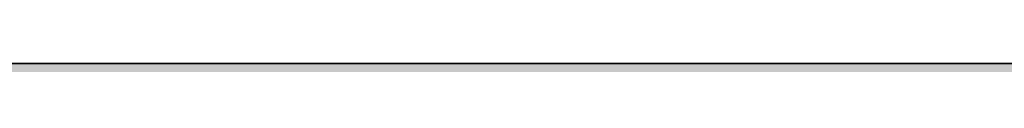
# Model space of a CAD drawing. Units: inches. Extents: x 2091 to 2899, y 967 to 2217.
# Tile 58 of 256: x 2212.16216 to 2212.20615, y 1099.919 to 1099.91906. Entities that reach past the tile are written whole.
import ezdxf

# ---------------------------------------------------------------- set-up
doc = ezdxf.new("R2010")
doc.units = ezdxf.units.IN
doc.layers.add('A-WALL-PATT', color=141, linetype='Continuous', lineweight=13, true_color=0xadddf7)
doc.layers.add('L-SITE-WALL', color=7, linetype='Continuous', lineweight=35)

msp = doc.modelspace()

# ---------------------------------------------------------------- hatches: boundary and pattern name
at = {"layer": 'A-WALL-PATT'}
h = msp.add_hatch(color=256, dxfattribs=at)
h.dxf.hatch_style = 1
h.paths.add_polyline_path([(2212.143603, 1941.419059), (2387.643603, 1941.419059), (2387.643603, 1824.419059), (2392.143603, 1824.419059), (2392.143603, 1941.419059), (2609.643603, 1941.419059), (2609.643603, 1825.919059), (2614.143603, 1825.919059), (2614.143603, 1941.419059), (2794.143603, 1941.419059), (2794.143603, 1928.762166), (2803.143603, 1928.762166), (2803.143603, 2050.919059), (2203.143603, 2050.919059), (2203.143603, 1900.757859), (2212.143603, 1900.757859)])
h.paths.add_polyline_path([(2212.143603, 1945.919059), (2212.143603, 2041.919059), (2794.143603, 2041.919059), (2794.143603, 1945.919059), (2402.248245, 1945.919059), (2401.102434, 1945.775832), (2398.702434, 1945.775832)], flags=16)
h.paths.add_polyline_path([(2230.229861, 1948.062793), (2227.349861, 1949.502793), (2225.909861, 1951.902793), (2223.989861, 1952.862793), (2223.029861, 1955.262793), (2222.069861, 1959.582793), (2222.069861, 1963.422793), (2223.029861, 1965.662793), (2223.989861, 1965.342793), (2225.58591, 1963.860747), (2226.911533, 1964.957259), (2226.948861, 1965.938793), (2227.778319, 1966.952143), (2228.199916, 1968.878704), (2230.709861, 1964.862793), (2233.589861, 1966.302793), (2233.607309, 1966.331873), (2233.772659, 1964.938205), (2234.633802, 1963.676473), (2235.029861, 1963.902793), (2236.282035, 1965.572358), (2235.989861, 1962.942793), (2237.954512, 1957.540002), (2238.389861, 1957.902793), (2239.215861, 1960.305793), (2238.654565, 1966.38496), (2238.692792, 1966.438069), (2238.840578, 1967.499707), (2238.780291, 1967.687486), (2238.880538, 1967.786763), (2238.666861, 1966.251793), (2239.215861, 1960.305793), (2238.389861, 1957.902793), (2236.949861, 1956.702793), (2234.549861, 1949.982793)], flags=0)
h.paths.add_polyline_path([(2278.011974, 1948.062793), (2276.496427, 1947.873349), (2275.849833, 1947.688608), (2274.651974, 1947.102793)], flags=0)
h.paths.add_polyline_path([(2269.851974, 1955.742793), (2268.276176, 1956.629329), (2270.867302, 1956.348398), (2269.371974, 1958.142793), (2268.714964, 1959.192325), (2270.569833, 1958.728608), (2268.580725, 1961.906087), (2270.811974, 1960.891883), (2270.811974, 1963.422793), (2271.393315, 1964.779256), (2270.291762, 1966.156196), (2271.771974, 1965.662793), (2272.141387, 1966.524757), (2273.929833, 1965.928608), (2275.630385, 1968.054299), (2276.331938, 1966.72186), (2276.520431, 1966.952143), (2276.942029, 1968.878704), (2277.734293, 1967.611082), (2278.139888, 1969.46452), (2279.659124, 1967.033742), (2280.411974, 1966.782793), (2280.949302, 1967.588785), (2281.609833, 1967.368608), (2282.133266, 1968.153758), (2282.349235, 1966.333445), (2282.349849, 1966.332585), (2283.40755, 1968.09542), (2283.712631, 1965.52402), (2284.320221, 1964.633789), (2284.511809, 1964.889239), (2284.234974, 1965.704793), (2284.500472, 1967.318958), (2284.907944, 1965.41742), (2285.396313, 1966.068579), (2285.432833, 1966.290608), (2285.473338, 1966.171279), (2286.353919, 1967.345387), (2286.222007, 1966.158173), (2287.663492, 1968.080154), (2287.713974, 1968.442793), (2288.481599, 1969.016679), (2288.573993, 1968.728897), (2288.917461, 1969.06904), (2288.606833, 1966.837608), (2288.928726, 1963.35131), (2288.934974, 1963.356793), (2288.929731, 1963.340422), (2289.015281, 1962.413869), (2290.111223, 1963.875126), (2290.132833, 1963.942608), (2290.217672, 1964.017058), (2290.111223, 1963.875126), (2289.155833, 1960.891608), (2288.594036, 1959.257227), (2288.571974, 1959.102793), (2289.531974, 1960.542793), (2290.011974, 1962.462793), (2290.19184, 1962.642659), (2289.769833, 1959.688608), (2286.889833, 1957.288608), (2284.489833, 1950.568608), (2283.314658, 1950.046308), (2283.291974, 1949.982793), (2280.290059, 1948.648608), (2281.129833, 1948.648608), (2282.569833, 1948.168608), (2283.204726, 1948.062793), (2278.971974, 1948.062793), (2276.091974, 1949.502793), (2274.651974, 1951.902793), (2272.731974, 1952.862793)], flags=0)
h.paths.add_polyline_path([(2271.158868, 1958.021765), (2272.969833, 1955.848608), (2272.009833, 1960.168608), (2272.009833, 1964.008608), (2272.624426, 1965.442658), (2274.328023, 1963.860747), (2275.653646, 1964.957259), (2275.637743, 1964.53909), (2277.412231, 1966.006888), (2277.032974, 1965.156793), (2276.829924, 1964.975597), (2276.766012, 1963.295014), (2277.449635, 1962.66022), (2279.451974, 1964.862793), (2282.331974, 1966.302793), (2283.529833, 1966.888608), (2283.294512, 1966.770948), (2283.912993, 1963.8847), (2284.899249, 1964.448275), (2284.731974, 1962.942793), (2286.696625, 1957.540002), (2287.131974, 1957.902793), (2287.541913, 1959.095388), (2287.779395, 1958.442311), (2285.682738, 1956.695097), (2285.876503, 1959.795336), (2284.731974, 1962.942793), (2284.899249, 1964.448275), (2283.912993, 1963.8847), (2284.223833, 1962.434116), (2283.424365, 1963.605484), (2281.609833, 1962.568608), (2281.129833, 1960.168608), (2282.089833, 1956.328608), (2283.049833, 1952.968608), (2282.569833, 1950.568608), (2280.169833, 1948.648608), (2279.883316, 1948.791867), (2278.971974, 1948.062793), (2278.971974, 1949.022793), (2278.672313, 1949.397368), (2277.289833, 1950.088608), (2275.849833, 1952.488608), (2273.929833, 1953.448608), (2272.489833, 1954.888608), (2271.921647, 1954.888608), (2271.771974, 1955.262793)], flags=0)
h.paths.add_polyline_path([(2311.994146, 1955.742793), (2312.062717, 1955.674221), (2312.0551, 1955.7085)], flags=0)
h.paths.add_polyline_path([(2331.956146, 1963.951793), (2333.396146, 1965.391793), (2331.077146, 1963.356793), (2330.998603, 1963.111517)], flags=0)
h.paths.add_polyline_path([(2310.554146, 1954.302793), (2307.039807, 1956.279943), (2310.762903, 1955.876284), (2312.474146, 1953.822793), (2313.434146, 1951.422793), (2315.354146, 1950.462793), (2316.794146, 1948.062793), (2317.466146, 1947.726793), (2319.368691, 1947.964611), (2317.754146, 1949.982793), (2317.569531, 1950.610485), (2316.794146, 1951.902793), (2314.874146, 1952.862793), (2313.914146, 1955.262793), (2311.514146, 1958.142793), (2309.375489, 1961.559168), (2311.514146, 1960.337078), (2311.514146, 1961.982793), (2310.604672, 1963.119635), (2311.726605, 1962.47853), (2312.418332, 1964.09256), (2312.255964, 1964.29552), (2313.194146, 1963.982793), (2313.914146, 1965.662793), (2314.646778, 1965.418582), (2315.354146, 1966.302793), (2316.794146, 1967.742793), (2316.157435, 1966.946904), (2317.034111, 1965.28186), (2317.222604, 1965.512143), (2317.777048, 1968.045771), (2318.474111, 1966.72186), (2318.662604, 1966.952143), (2319.084201, 1968.878704), (2321.207049, 1965.482147), (2322.161419, 1966.913702), (2322.554146, 1966.782793), (2322.785988, 1967.130555), (2322.881646, 1966.324293), (2323.312041, 1965.72174), (2323.651289, 1965.891364), (2324.3965, 1967.133382), (2324.656945, 1964.938205), (2324.971986, 1964.476611), (2325.38728, 1967.001499), (2325.940813, 1964.418348), (2327.228929, 1966.135836), (2327.16632, 1965.572358), (2328.059139, 1966.762783), (2328.224576, 1966.247486), (2329.667971, 1967.67691), (2329.664576, 1967.687486), (2329.764823, 1967.786763), (2329.551146, 1966.251793), (2330.100146, 1960.305793), (2329.332814, 1958.07347), (2329.313065, 1957.935225), (2329.634146, 1958.202793), (2330.234146, 1959.102793), (2330.714146, 1961.022793), (2331.034146, 1961.342793), (2330.714146, 1959.102793), (2329.634146, 1958.202793), (2329.274146, 1957.662793), (2327.712112, 1956.361098), (2325.434146, 1949.982793), (2324.333769, 1949.493736), (2323.994146, 1948.542793), (2319.674146, 1946.622793), (2316.794146, 1948.062793), (2315.354146, 1950.462793), (2313.434146, 1951.422793)], flags=0)
h.paths.add_polyline_path([(2321.335684, 1947.952023), (2321.114146, 1948.062793), (2321.114146, 1949.022793), (2319.194146, 1951.422793), (2316.794146, 1959.582793), (2316.663237, 1959.582793), (2315.354146, 1958.142793), (2314.394146, 1958.142793), (2313.148303, 1958.709085), (2312.954146, 1959.582793), (2312.954146, 1960.891883), (2315.834146, 1959.582793), (2316.663237, 1959.582793), (2317.314709, 1960.299412), (2315.030195, 1962.420747), (2316.355818, 1963.517259), (2316.372337, 1963.951615), (2316.470195, 1963.860747), (2317.795818, 1964.957259), (2317.755219, 1963.889687), (2319.175146, 1965.156793), (2319.498407, 1965.881372), (2321.114146, 1965.342793), (2323.235885, 1962.372358), (2325.686349, 1963.772623), (2325.542789, 1962.480576), (2325.198783, 1963.494014), (2324.47851, 1963.082429), (2324.926005, 1960.994116), (2324.078087, 1962.236473), (2322.414791, 1961.286018), (2322.074146, 1959.582793), (2323.034146, 1955.742793), (2323.994146, 1952.382793), (2323.514146, 1949.982793), (2322.142717, 1948.88565), (2322.074146, 1948.542793)], flags=0)
h.paths.add_polyline_path([(2320.207479, 1963.337459), (2320.154146, 1963.422793), (2320.394146, 1963.542793)], flags=0)
h.paths.add_polyline_path([(2353.850527, 1965.8105), (2354.030527, 1965.7505), (2354.330527, 1966.4505), (2354.330527, 1966.9305)], flags=0)
h.paths.add_polyline_path([(2359.020582, 1969.026412), (2359.098382, 1968.901932), (2359.233527, 1969.5195), (2359.233527, 1969.9995)], flags=0)
h.paths.add_polyline_path([(2358.256694, 1966.681672), (2357.983601, 1966.348035), (2358.211267, 1966.146175), (2358.410492, 1966.389568)], flags=0)
h.paths.add_polyline_path([(2357.768473, 1966.058778), (2357.7322, 1965.104967), (2357.751047, 1965.120556), (2357.769527, 1965.6065), (2357.769527, 1966.057843)], flags=0)
h.paths.add_polyline_path([(2359.111527, 1965.3045), (2359.111527, 1964.8245), (2359.844527, 1966.4675), (2359.844527, 1966.9475)], flags=0)
h.paths.add_polyline_path([(2360.223684, 1966.621449), (2360.698527, 1969.3625), (2360.698527, 1969.8425), (2360.210527, 1967.0255), (2360.210527, 1966.6425)], flags=0)
h.paths.add_polyline_path([(2363.450527, 1967.8905), (2363.450527, 1968.3705), (2362.490527, 1966.9305), (2362.656045, 1966.698776)], flags=0)
h.paths.add_polyline_path([(2364.475523, 1966.078826), (2365.850527, 1968.3705), (2365.850527, 1968.8505), (2364.427975, 1966.479581)], flags=0)
h.paths.add_polyline_path([(2366.313527, 1965.8525), (2366.366709, 1965.695829), (2366.802527, 1968.3455), (2366.802527, 1968.8255)], flags=0)
h.paths.add_polyline_path([(2367.16531, 1965.803544), (2367.290527, 1966.9305), (2367.290527, 1967.4105), (2367.102701, 1965.720066)], flags=0)
h.paths.add_polyline_path([(2370.036527, 1959.9735), (2371.013527, 1963.0245), (2371.013527, 1963.5045), (2370.036527, 1960.4535)], flags=0)
h.paths.add_polyline_path([(2371.610527, 1960.2105), (2372.570527, 1961.6505), (2372.570527, 1962.1305), (2371.802527, 1960.9785)], flags=0)
h.paths.add_polyline_path([(2350.873666, 1956.005086), (2351.930527, 1955.8905), (2354.490527, 1953.3305), (2353.850527, 1954.9305), (2351.450527, 1957.8105), (2347.935527, 1963.4255), (2347.935527, 1963.9055), (2351.450527, 1958.2905), (2353.705073, 1955.585046), (2352.890527, 1959.2505), (2352.890527, 1959.7305), (2352.890527, 1961.924786), (2356.730527, 1959.7305), (2358.454471, 1961.626838), (2354.810527, 1965.0105), (2355.030855, 1965.28591), (2358.691091, 1961.88712), (2361.530527, 1965.0105), (2364.376495, 1966.433484), (2364.524394, 1965.186911), (2365.454468, 1963.824181), (2365.881073, 1964.067955), (2365.370527, 1966.4505), (2365.370527, 1966.9305), (2366.810527, 1960.2105), (2366.810527, 1959.7305), (2366.388709, 1952.981409), (2367.770527, 1956.8505), (2368.641225, 1957.576082), (2366.810527, 1962.6105), (2366.810527, 1963.0905), (2368.775179, 1957.68771), (2369.210527, 1958.0505), (2370.001592, 1960.351867), (2369.475232, 1966.052668), (2369.513458, 1966.105777), (2369.514173, 1966.110912), (2369.475232, 1966.532668), (2369.513458, 1966.585777), (2369.614635, 1967.312591), (2369.182527, 1968.6585), (2369.182527, 1969.1385), (2369.600957, 1967.835194), (2369.701204, 1967.934471), (2369.717947, 1968.054743), (2370.145176, 1968.374145), (2369.778707, 1968.011224), (2369.701204, 1967.454471), (2370.468161, 1968.214004), (2369.674936, 1967.265771), (2369.514173, 1966.110912), (2370.036527, 1960.4535), (2370.036527, 1959.9735), (2369.441756, 1958.243191), (2370.650527, 1959.2505), (2371.045821, 1962.017559), (2371.130527, 1962.1305), (2370.650527, 1958.7705), (2367.770527, 1956.3705), (2365.370527, 1949.6505), (2362.079099, 1948.187643), (2363.450527, 1947.7305), (2361.050527, 1947.7305), (2360.090527, 1947.7305), (2357.103861, 1947.357167), (2360.090527, 1948.2105), (2358.170527, 1949.1705), (2356.730527, 1951.5705), (2354.810527, 1952.5305), (2351.930527, 1955.4105)], flags=0)
h.paths.add_polyline_path([(2361.050527, 1948.6905), (2359.130527, 1951.0905), (2356.730527, 1959.2505), (2355.770527, 1959.2505), (2352.890527, 1960.559591), (2352.890527, 1961.444786), (2355.890527, 1959.7305), (2356.730527, 1959.7305), (2356.837194, 1959.367834), (2361.530527, 1964.5305), (2363.248422, 1965.389448), (2364.92531, 1963.041805), (2362.490527, 1961.6505), (2362.063861, 1959.517167), (2362.970527, 1955.8905), (2363.930527, 1952.5305), (2363.930527, 1952.0505), (2363.450527, 1949.6505), (2361.050527, 1947.7305)], flags=0)
h.paths.add_polyline_path([(2359.130527, 1951.5705), (2359.290527, 1951.3705), (2361.050527, 1954.4505), (2361.050527, 1954.9305)], flags=0)
h.paths.add_polyline_path([(2357.219527, 1966.5455), (2356.792527, 1968.8145), (2356.792527, 1969.2945), (2357.219527, 1967.0255)], flags=0)
h.paths.add_polyline_path([(2361.050527, 1954.4505), (2361.530527, 1958.7705), (2361.530527, 1959.2505), (2361.050527, 1954.9305)], flags=0)
h.paths.add_polyline_path([(2402.548287, 1948.486076), (2402.302434, 1948.415832), (2402.590434, 1948.415832)], flags=0)
h.paths.add_polyline_path([(2394.142434, 1956.095832), (2395.685052, 1954.553214), (2396.720495, 1953.970679), (2396.062434, 1955.615832), (2395.241381, 1956.601096), (2395.878904, 1956.441715), (2395.102434, 1959.935832), (2395.102434, 1963.775832), (2396.062434, 1966.015832), (2397.022434, 1965.695832), (2398.618483, 1964.213787), (2399.944106, 1965.310299), (2399.981434, 1966.291832), (2400.810891, 1967.305183), (2401.232489, 1969.231744), (2403.537949, 1965.543008), (2403.941984, 1967.389316), (2404.702434, 1967.135832), (2405.460328, 1966.07478), (2406.622434, 1966.655832), (2406.639882, 1966.684913), (2406.805232, 1965.291245), (2406.925694, 1965.114746), (2407.342434, 1964.975832), (2407.874326, 1965.77367), (2408.1691, 1964.398055), (2409.314608, 1965.925398), (2409.217458, 1965.051054), (2409.445232, 1963.131245), (2410.306374, 1961.869513), (2410.702434, 1962.095832), (2411.442269, 1963.082279), (2411.165434, 1963.897832), (2411.616426, 1966.639757), (2411.725365, 1966.791109), (2411.873151, 1967.852747), (2411.812864, 1968.040526), (2411.913111, 1968.139803), (2411.699434, 1966.604832), (2412.248434, 1960.658832), (2413.225434, 1963.709832), (2414.3779, 1964.72116), (2414.513151, 1965.692747), (2414.452864, 1965.880526), (2414.553111, 1965.979803), (2414.3779, 1964.72116), (2414.519817, 1964.845697), (2414.365365, 1964.631109), (2414.339434, 1964.444832), (2414.888434, 1958.498832), (2414.062434, 1956.095832), (2412.622434, 1954.895832), (2410.17137, 1948.032854), (2410.016719, 1948.084404), (2405.902434, 1946.255832), (2405.902434, 1947.215832), (2405.204252, 1948.08856), (2404.222434, 1948.415832), (2403.262434, 1948.415832), (2400.382434, 1949.855832), (2399.662434, 1951.055832), (2397.982434, 1952.735832), (2397.022434, 1953.215832), (2395.685052, 1954.553214), (2392.656776, 1956.256908)], flags=0)
h.paths.add_polyline_path([(2409.08565, 1964.407441), (2409.130363, 1964.275715), (2409.262434, 1964.495832)], flags=0)
h.paths.add_polyline_path([(2397.742434, 1961.615832), (2398.702434, 1963.855832), (2399.662434, 1963.535832), (2401.426563, 1965.740994), (2401.791415, 1966.5588), (2402.071434, 1965.070832), (2402.835507, 1964.393367), (2403.262398, 1964.9149), (2403.338119, 1964.771086), (2402.615516, 1963.976223), (2402.498612, 1960.902238), (2403.542997, 1959.932452), (2404.413203, 1960.889679), (2404.702434, 1962.335832), (2407.916347, 1964.172354), (2409.520211, 1961.926944), (2410.987085, 1957.893042), (2411.422434, 1958.255832), (2412.047964, 1960.075625), (2412.410341, 1959.079088), (2411.675621, 1958.466821), (2411.662434, 1958.255832), (2411.62607, 1958.425529), (2409.982434, 1957.055832), (2407.582434, 1950.335832), (2403.262434, 1948.415832), (2403.262434, 1949.375832), (2401.342434, 1951.775832), (2399.416508, 1958.323981), (2397.742434, 1959.084923), (2397.742434, 1959.970118), (2397.102434, 1960.335832), (2397.742434, 1960.044923)], flags=0)
h.paths.add_polyline_path([(2405.902434, 1952.975832), (2405.950434, 1953.407832), (2406.016719, 1953.175832)], flags=0)
h.paths.add_polyline_path([(2449.817778, 1967.114014), (2449.752323, 1967.135832), (2449.793703, 1967.077901)], flags=0)
h.paths.add_polyline_path([(2451.697696, 1966.61812), (2451.740895, 1966.690118), (2451.692051, 1966.665696)], flags=0)
h.paths.add_polyline_path([(2454.343628, 1965.737572), (2455.752323, 1967.615832), (2455.992323, 1968.095832), (2454.364497, 1965.925398)], flags=0)
h.paths.add_polyline_path([(2457.547323, 1968.863832), (2457.787323, 1969.343832), (2457.054323, 1968.795832), (2457.007622, 1968.460345)], flags=0)
h.paths.add_polyline_path([(2456.921784, 1967.856662), (2456.802238, 1968.229016), (2456.723, 1967.659803)], flags=0)
h.paths.add_polyline_path([(2457.302323, 1967.376832), (2457.542323, 1967.856832), (2456.810323, 1966.839832), (2456.740516, 1966.700218), (2456.749021, 1966.608105)], flags=0)
h.paths.add_polyline_path([(2458.275323, 1963.709832), (2458.155343, 1963.335153), (2460.354323, 1965.264832), (2460.594323, 1965.744832)], flags=0)
h.paths.add_polyline_path([(2458.392323, 1962.815832), (2458.364088, 1962.618185), (2459.592323, 1964.255832), (2459.832323, 1964.735832)], flags=0)
h.paths.add_polyline_path([(2459.352323, 1962.815832), (2459.272323, 1962.495832), (2460.072323, 1963.295832), (2460.312323, 1963.775832)], flags=0)
h.paths.add_polyline_path([(2458.680323, 1960.607832), (2458.632323, 1960.415832), (2459.592323, 1961.855832), (2459.832323, 1962.335832)], flags=0)
h.paths.add_polyline_path([(2437.83817, 1956.24265), (2439.192323, 1956.095832), (2441.352323, 1953.935832), (2440.872323, 1955.135832), (2438.472323, 1958.015832), (2438.071563, 1958.656023), (2438.712323, 1958.495832), (2440.639596, 1956.183105), (2439.912323, 1959.455832), (2439.912323, 1963.295832), (2441.352323, 1966.655832), (2441.592323, 1967.135832), (2441.112323, 1966.015832), (2442.072323, 1965.695832), (2443.988993, 1968.09167), (2444.241323, 1966.750832), (2444.916801, 1966.15192), (2445.676574, 1967.080136), (2446.255323, 1969.724832), (2446.495323, 1970.204832), (2446.282379, 1969.231744), (2447.362672, 1967.503275), (2447.720323, 1969.567832), (2447.960323, 1970.047832), (2447.48548, 1967.306781), (2448.792323, 1965.215832), (2448.472323, 1964.863832), (2448.552323, 1964.735832), (2451.452051, 1966.185696), (2451.615122, 1964.811245), (2452.307917, 1963.796172), (2453.234505, 1964.325651), (2454.072323, 1960.415832), (2453.628687, 1953.317651), (2454.792323, 1956.575832), (2455.032323, 1957.055832), (2455.718835, 1957.627926), (2453.832323, 1962.815832), (2453.940966, 1963.793615), (2453.335323, 1965.577832), (2453.824323, 1968.550832), (2454.064323, 1969.030832), (2453.575323, 1966.057832), (2454.040333, 1964.687919), (2453.832323, 1962.815832), (2455.718835, 1957.627926), (2456.367207, 1958.168235), (2457.058323, 1960.178832), (2457.298323, 1960.658832), (2456.472323, 1958.255832), (2457.717729, 1959.29367), (2457.672323, 1958.975832), (2454.889951, 1956.657188), (2453.614142, 1953.084923), (2453.592323, 1952.735832), (2453.352323, 1952.255832), (2453.359596, 1952.372196), (2452.632323, 1950.335832), (2452.392323, 1949.855832), (2449.203752, 1948.43869), (2450.712323, 1947.935832), (2448.072323, 1947.935832), (2447.112323, 1947.935832), (2444.552323, 1947.615832), (2447.199596, 1948.372196), (2445.192323, 1949.375832), (2443.752323, 1951.775832), (2441.832323, 1952.735832), (2438.952323, 1955.615832)], flags=0)
h.paths.add_polyline_path([(2443.992323, 1959.935832), (2444.040323, 1959.772632), (2444.121554, 1959.861986)], flags=0)
h.paths.add_polyline_path([(2442.912323, 1959.935832), (2443.032323, 1959.935832), (2442.445657, 1960.202499)], flags=0)
h.paths.add_polyline_path([(2444.982943, 1965.019677), (2445.279323, 1965.264832), (2445.519323, 1965.744832), (2444.993996, 1965.310299)], flags=0)
h.paths.add_polyline_path([(2446.133323, 1965.029832), (2446.330366, 1965.471499), (2444.970323, 1964.257832), (2444.730323, 1963.777832)], flags=0)
h.paths.add_polyline_path([(2442.792323, 1959.455832), (2443.752323, 1959.455832), (2446.152323, 1951.295832), (2446.412323, 1951.750832), (2446.392323, 1951.775832), (2448.080599, 1954.730315), (2448.552323, 1958.975832), (2441.832323, 1965.215832), (2442.154946, 1965.619111), (2448.792323, 1959.455832), (2448.312323, 1955.135832), (2448.072323, 1954.655832), (2446.412323, 1951.750832), (2448.312323, 1949.375832), (2448.312323, 1948.415832), (2450.540895, 1950.19869), (2450.952323, 1952.255832), (2449.992323, 1955.615832), (2449.032323, 1959.455832), (2449.512323, 1961.855832), (2449.752323, 1962.335832), (2449.674904, 1961.948736), (2452.994505, 1963.845651), (2453.064414, 1963.519409), (2452.884611, 1963.782854), (2449.674904, 1961.948736), (2449.272323, 1959.935832), (2450.232323, 1956.095832), (2451.192323, 1952.735832), (2450.712323, 1950.335832), (2450.472323, 1949.855832), (2448.072323, 1947.935832), (2448.072323, 1948.535832), (2445.432323, 1949.855832), (2443.992323, 1952.255832), (2442.072323, 1953.215832), (2441.112323, 1955.615832), (2440.152323, 1959.935832), (2440.152323, 1960.655832)], flags=0)
h.paths.add_polyline_path([(2456.692323, 1966.985832), (2457.608323, 1968.080832), (2457.848323, 1968.560832), (2456.932323, 1967.465832)], flags=0)
h.paths.add_polyline_path([(2489.89657, 1966.580241), (2489.942948, 1966.189347), (2490.747488, 1967.530248), (2491.319122, 1968.951161)], flags=0)
h.paths.add_polyline_path([(2473.562471, 1956.407131), (2477.139981, 1956.019257), (2476.955333, 1956.240834), (2475.108049, 1957.280108), (2476.347488, 1956.970248), (2475.186901, 1958.824216), (2476.919122, 1958.391161), (2475.411642, 1960.799269), (2477.787488, 1959.719339), (2477.787488, 1962.250248), (2477.637399, 1962.43786), (2477.82255, 1962.332059), (2478.359122, 1963.58406), (2478.359122, 1963.671161), (2477.324348, 1964.964628), (2478.714826, 1964.501135), (2479.319122, 1965.911161), (2480.279122, 1965.591161), (2481.783965, 1967.472214), (2482.116488, 1965.705248), (2482.880562, 1965.027782), (2483.209305, 1965.429408), (2483.220169, 1965.71509), (2483.07594, 1965.989022), (2483.711762, 1966.765808), (2484.130488, 1968.679248), (2484.702122, 1970.100161), (2484.489177, 1969.127072), (2486.502904, 1965.905109), (2487.387488, 1965.610248), (2488.153419, 1966.759144), (2488.717017, 1965.970108), (2489.200086, 1966.211642), (2489.330671, 1965.110992), (2490.393905, 1963.622465), (2490.660765, 1963.774956), (2490.493905, 1964.553636), (2490.923063, 1963.924841), (2491.319122, 1964.151161), (2491.333389, 1964.170183), (2491.210488, 1964.532248), (2491.281756, 1964.965537), (2491.425789, 1964.293383), (2494.076476, 1967.827632), (2494.497918, 1966.514942), (2494.598165, 1966.614218), (2494.689488, 1967.270248), (2495.106748, 1967.582196), (2495.129839, 1967.748075), (2495.069552, 1967.935854), (2495.169799, 1968.035131), (2495.031777, 1967.043632), (2495.753818, 1967.758684), (2494.982053, 1966.686437), (2494.956122, 1966.500161), (2495.479021, 1960.836851), (2495.910488, 1962.184248), (2496.482122, 1963.605161), (2496.072694, 1962.326589), (2496.768904, 1962.937536), (2496.599122, 1962.711161), (2496.119122, 1959.351161), (2496.732873, 1960.271787), (2496.987488, 1961.290248), (2497.559122, 1962.711161), (2497.079122, 1960.791161), (2496.507488, 1959.370248), (2495.547488, 1957.930248), (2492.758842, 1955.606376), (2490.839122, 1950.231161), (2490.267488, 1948.810248), (2485.947488, 1946.890248), (2483.067488, 1948.330248), (2481.627488, 1950.730248), (2479.707488, 1951.690248), (2476.827488, 1954.570248)], flags=0)
h.paths.add_polyline_path([(2485.576973, 1948.313392), (2485.559122, 1948.311161), (2485.578758, 1948.311161)], flags=0)
h.paths.add_polyline_path([(2478.645063, 1954.551161), (2478.109042, 1956.963257), (2479.319122, 1955.511161), (2480.279122, 1953.111161), (2482.199122, 1952.151161), (2483.639122, 1949.751161), (2486.519122, 1948.311161), (2486.519122, 1949.271161), (2484.739307, 1951.49593), (2484.027488, 1950.250248), (2481.627488, 1958.410248), (2482.375148, 1959.232673), (2482.199122, 1959.831161), (2483.197572, 1960.929456), (2479.707488, 1964.170248), (2480.603358, 1965.290085), (2481.875171, 1964.109115), (2482.666387, 1964.763582), (2482.615359, 1963.421798), (2482.989199, 1963.074661), (2484.008488, 1963.984248), (2484.683606, 1965.497507), (2484.580122, 1965.405161), (2485.357268, 1967.147113), (2485.120645, 1965.781197), (2486.427488, 1963.690248), (2488.145383, 1964.549195), (2489.822271, 1962.201552), (2490.747488, 1962.730248), (2491.999662, 1964.399813), (2492.076046, 1965.087265), (2492.212892, 1964.684119), (2492.485374, 1965.047429), (2492.279122, 1963.191161), (2494.243773, 1957.78837), (2494.562503, 1958.053978), (2494.933488, 1959.133248), (2495.505122, 1960.554161), (2494.679122, 1958.151161), (2494.107488, 1956.730248), (2494.562503, 1958.053978), (2493.408544, 1957.092345), (2491.707488, 1961.770248), (2491.999662, 1964.399813), (2490.747488, 1962.730248), (2487.71203, 1960.9957), (2487.479122, 1959.831161), (2488.439122, 1955.991161), (2489.399122, 1952.631161), (2488.919122, 1950.231161), (2488.576918, 1949.957397), (2488.347488, 1948.810248), (2487.651715, 1948.253629), (2487.479122, 1948.311161), (2486.519122, 1948.311161), (2483.639122, 1949.751161), (2482.199122, 1952.151161), (2480.279122, 1953.111161), (2478.839122, 1954.551161)], flags=0)
h.paths.add_polyline_path([(2526.648252, 1966.987524), (2526.517343, 1967.031161), (2526.600102, 1966.915298)], flags=0)
h.paths.add_polyline_path([(2528.47064, 1966.446656), (2528.574486, 1966.619732), (2528.457071, 1966.561025)], flags=0)
h.paths.add_polyline_path([(2534.133343, 1967.496161), (2534.156685, 1967.542845), (2534.059841, 1967.408296)], flags=0)
h.paths.add_polyline_path([(2536.161923, 1964.0506), (2535.157343, 1962.711161), (2535.100872, 1962.315866), (2536.117343, 1963.671161), (2536.420532, 1964.277539)], flags=0)
h.paths.add_polyline_path([(2535.157343, 1959.831161), (2536.117343, 1961.271161), (2536.597343, 1962.231161), (2535.253343, 1960.215161)], flags=0)
h.paths.add_polyline_path([(2513.249035, 1956.284796), (2516.221181, 1955.962555), (2514.997343, 1957.431161), (2514.195823, 1958.711541), (2515.477343, 1958.391161), (2516.931888, 1956.645706), (2516.437343, 1958.871161), (2516.437343, 1962.711161), (2516.872692, 1963.726974), (2515.346434, 1965.634797), (2517.397343, 1964.951161), (2517.877343, 1966.071161), (2518.357343, 1967.031161), (2517.877343, 1965.911161), (2518.837343, 1965.591161), (2520.48659, 1967.652719), (2520.766343, 1966.166161), (2521.530417, 1965.488695), (2521.781443, 1965.795375), (2521.800911, 1966.307268), (2521.477804, 1966.920936), (2521.246343, 1967.126161), (2521.177701, 1967.490913), (2521.477804, 1966.920936), (2522.010417, 1966.448695), (2522.257386, 1966.750417), (2522.780343, 1969.140161), (2523.260343, 1970.100161), (2523.047398, 1969.127072), (2524.673132, 1966.525897), (2526.037343, 1966.071161), (2526.795238, 1965.010108), (2527.977071, 1965.601025), (2528.140141, 1964.226573), (2528.66459, 1963.458159), (2529.388616, 1963.871888), (2529.329665, 1964.14699), (2529.481284, 1963.924841), (2529.877343, 1964.151161), (2529.98401, 1964.293383), (2529.789053, 1965.20318), (2530.0624, 1964.397903), (2532.802483, 1968.051347), (2533.147773, 1966.975854), (2533.24802, 1967.075131), (2533.339343, 1967.731161), (2533.672848, 1967.980493), (2533.72802, 1968.035131), (2533.514343, 1966.500161), (2534.024718, 1960.972496), (2534.560343, 1962.645161), (2535.040343, 1963.605161), (2534.063343, 1960.554161), (2533.237343, 1958.151161), (2534.288154, 1959.026836), (2534.197343, 1958.391161), (2531.512597, 1956.153872), (2529.397343, 1950.231161), (2528.917343, 1949.271161), (2526.448772, 1948.174018), (2527.477343, 1947.831161), (2530.357343, 1947.351161), (2524.597343, 1947.351161), (2521.717343, 1948.791161), (2520.277343, 1951.191161), (2518.357343, 1952.151161), (2515.477343, 1955.031161)], flags=0)
h.paths.add_polyline_path([(2523.93476, 1967.190308), (2523.619512, 1966.483689), (2523.7705, 1966.242109)], flags=0)
h.paths.add_polyline_path([(2518.837343, 1953.111161), (2517.877343, 1955.511161), (2516.884983, 1959.976779), (2516.917343, 1959.96207), (2516.917343, 1962.025446), (2520.757343, 1959.831161), (2522.024949, 1961.225527), (2518.357343, 1964.631161), (2519.002589, 1965.437718), (2520.433392, 1964.109115), (2521.30112, 1964.826871), (2521.245157, 1963.355333), (2525.638307, 1959.27598), (2526.037343, 1961.271161), (2529.397343, 1963.191161), (2530.649517, 1964.860726), (2530.66472, 1964.99755), (2530.691956, 1964.917311), (2531.087778, 1965.445074), (2530.945985, 1964.168944), (2530.691956, 1964.917311), (2529.397343, 1963.191161), (2526.362504, 1961.456967), (2526.037343, 1959.831161), (2526.997343, 1955.991161), (2527.957343, 1952.631161), (2527.477343, 1950.231161), (2527.134486, 1949.956875), (2526.973928, 1949.154087), (2526.697343, 1949.031161), (2524.597343, 1947.351161), (2524.597343, 1948.311161), (2524.277343, 1948.711161), (2522.197343, 1949.751161), (2520.757343, 1952.151161)], flags=0)
h.paths.add_polyline_path([(2520.277343, 1958.871161), (2520.853343, 1959.504761), (2523.157343, 1951.671161), (2524.613895, 1954.220126), (2524.597343, 1954.071161), (2522.677343, 1950.711161)], flags=0)
h.paths.add_polyline_path([(2559.37091, 1966.311161), (2559.398411, 1966.324911), (2559.401943, 1966.345296)], flags=0)
h.paths.add_polyline_path([(2549.77091, 1957.191161), (2552.65091, 1954.311161), (2552.133987, 1955.603468), (2550.61091, 1957.431161), (2547.09591, 1963.046161), (2545.77591, 1965.206161), (2549.29091, 1959.591161), (2551.69091, 1956.711161), (2550.792933, 1960.752059), (2550.73091, 1960.780251), (2550.73091, 1964.871161), (2551.69091, 1967.111161), (2552.65091, 1966.791161), (2554.246959, 1965.309115), (2555.034252, 1965.960337), (2555.581671, 1966.644612), (2555.60991, 1967.387161), (2556.439368, 1968.400511), (2556.860966, 1970.327072), (2559.37091, 1966.311161), (2560.69091, 1964.151161), (2562.408805, 1965.010108), (2561.65091, 1966.071161), (2560.33091, 1968.231161), (2561.758497, 1966.23254), (2562.347213, 1967.115614), (2562.433709, 1966.386573), (2563.127798, 1965.369604), (2563.57091, 1965.591161), (2563.588359, 1965.620241), (2563.362543, 1967.52354), (2563.722489, 1965.843792), (2565.060001, 1968.072979), (2564.732862, 1965.128722), (2565.117577, 1963.333383), (2567.444622, 1966.436109), (2567.315615, 1967.833328), (2567.353841, 1967.886437), (2567.501627, 1968.948075), (2567.44134, 1969.135854), (2567.541587, 1969.235131), (2567.32791, 1967.700161), (2567.87691, 1961.754161), (2568.746689, 1964.470327), (2568.635615, 1965.673328), (2568.673841, 1965.726437), (2568.821627, 1966.788075), (2568.76134, 1966.975854), (2568.861587, 1967.075131), (2568.64791, 1965.540161), (2568.726127, 1964.693026), (2568.85391, 1964.805161), (2568.746689, 1964.470327), (2568.817236, 1963.706261), (2568.97091, 1963.911161), (2568.866075, 1963.17731), (2569.19691, 1959.594161), (2568.37091, 1957.191161), (2566.93091, 1955.991161), (2564.620272, 1949.521373), (2564.65091, 1949.511161), (2564.616625, 1949.511161), (2564.53091, 1949.271161), (2560.21091, 1947.351161), (2557.33091, 1948.791161), (2556.045196, 1950.934018), (2556.01091, 1950.951161), (2555.856625, 1951.208303), (2553.97091, 1952.151161), (2551.09091, 1955.031161), (2546.650144, 1957.529515)], flags=0)
h.paths.add_polyline_path([(2567.025794, 1959.33023), (2567.035007, 1959.304895), (2567.05091, 1959.351161)], flags=0)
h.paths.add_polyline_path([(2551.968287, 1962.518374), (2553.01091, 1964.951161), (2553.97091, 1964.631161), (2555.566959, 1963.149115), (2556.892583, 1964.245627), (2556.92991, 1965.227161), (2557.143984, 1965.488695), (2556.420066, 1966.130557), (2556.391421, 1966.104995), (2556.37991, 1966.166161), (2556.420066, 1966.130557), (2556.95191, 1966.605161), (2557.092139, 1966.919478), (2557.570875, 1966.010228), (2557.759368, 1966.240511), (2557.41791, 1964.680161), (2556.892583, 1964.245627), (2556.807089, 1961.997566), (2560.69091, 1958.391161), (2560.635526, 1957.892699), (2560.81091, 1957.191161), (2561.77091, 1953.831161), (2561.29091, 1951.431161), (2559.110423, 1949.68677), (2559.156484, 1949.629193), (2563.02652, 1951.349209), (2562.61091, 1949.271161), (2560.21091, 1947.351161), (2560.21091, 1948.311161), (2559.25091, 1949.511161), (2558.89091, 1949.511161), (2558.89091, 1949.961161), (2558.29091, 1950.711161), (2558.053701, 1951.517672), (2556.97091, 1952.871161), (2555.06788, 1959.341464), (2552.05091, 1961.065446), (2552.05091, 1962.471161)], flags=0)
h.paths.add_polyline_path([(2588.330049, 1958.391161), (2588.610248, 1958.110962), (2588.553362, 1958.366949)], flags=0)
h.paths.add_polyline_path([(2594.745454, 1950.493086), (2593.957532, 1953.172022), (2593.130049, 1954.551161), (2591.210049, 1955.511161), (2590.250049, 1957.911161), (2588.309033, 1960.240379), (2586.177306, 1961.209346), (2587.850049, 1960.791161), (2587.253416, 1961.744246), (2588.441314, 1961.065446), (2588.441314, 1962.655528), (2588.421679, 1962.665345), (2588.441314, 1962.711161), (2586.914038, 1964.620256), (2588.877086, 1963.727962), (2589.290049, 1964.69154), (2589.290049, 1966.071161), (2590.250049, 1968.311161), (2591.210049, 1967.991161), (2592.806098, 1966.509115), (2594.131721, 1967.605627), (2594.169049, 1968.587161), (2594.998506, 1969.600511), (2595.420104, 1971.527072), (2597.930049, 1967.511161), (2600.810049, 1968.951161), (2600.827497, 1968.980241), (2600.992847, 1967.586573), (2601.853989, 1966.324841), (2602.107143, 1966.4695), (2602.236354, 1967.255069), (2602.356715, 1966.693383), (2603.502223, 1968.220726), (2603.210049, 1965.591161), (2605.1747, 1960.18837), (2605.506891, 1960.465196), (2605.026019, 1965.673328), (2605.064245, 1965.726437), (2605.212031, 1966.788075), (2605.151744, 1966.975854), (2605.251991, 1967.075131), (2605.343314, 1967.731161), (2605.952905, 1968.186898), (2605.874753, 1969.033328), (2605.912979, 1969.086437), (2606.060766, 1970.148075), (2606.000479, 1970.335854), (2606.100725, 1970.435131), (2605.887049, 1968.900161), (2606.436049, 1962.954161), (2605.610049, 1960.551161), (2605.997036, 1960.87365), (2606.564314, 1962.645161), (2608.241494, 1964.116941), (2608.010049, 1963.191161), (2607.050049, 1961.751161), (2606.631486, 1961.402358), (2606.201314, 1958.391161), (2603.321314, 1955.991161), (2600.921314, 1949.271161), (2596.601314, 1947.351161), (2593.721314, 1948.791161), (2592.857314, 1950.231161), (2592.650049, 1950.231161)], flags=0)
h.paths.add_polyline_path([(2596.601314, 1947.351161), (2596.601314, 1948.311161), (2594.681314, 1950.711161), (2596.154954, 1953.290029), (2595.530049, 1954.071161), (2593.199226, 1961.995957), (2592.65134, 1962.504708), (2591.780151, 1963.002531), (2593.282987, 1964.245627), (2593.320314, 1965.227161), (2594.149772, 1966.240511), (2594.57137, 1968.167072), (2596.182651, 1965.589023), (2596.951273, 1966.434508), (2598.041314, 1966.071161), (2598.799209, 1965.010108), (2599.961314, 1965.591161), (2599.978763, 1965.620241), (2600.144113, 1964.226573), (2601.005255, 1962.964841), (2601.401314, 1963.191161), (2602.653488, 1964.860726), (2602.361314, 1962.231161), (2603.792748, 1958.294719), (2601.977644, 1953.212427), (2601.946208, 1952.709453), (2599.468755, 1951.608363), (2599.001314, 1949.271161)], flags=0)
h.paths.add_polyline_path([(2597.561314, 1958.871161), (2597.670966, 1959.419419), (2597.595054, 1958.736204)], flags=0)
h.paths.add_polyline_path([(2623.666305, 1961.254375), (2625.519163, 1960.791161), (2624.965544, 1961.675533), (2627.199163, 1960.660251), (2627.199163, 1961.151161), (2626.959163, 1962.231161), (2626.959163, 1963.491161), (2625.582321, 1965.212213), (2626.959163, 1964.425446), (2626.959163, 1965.831161), (2626.869163, 1965.861161), (2627.919163, 1968.311161), (2628.879163, 1967.991161), (2630.475212, 1966.509115), (2631.800835, 1967.605627), (2631.838163, 1968.587161), (2632.667621, 1969.600511), (2633.089218, 1971.527072), (2635.599163, 1967.511161), (2638.479163, 1968.951161), (2638.496611, 1968.980241), (2638.661961, 1967.586573), (2639.176273, 1966.833011), (2639.780216, 1967.839582), (2640.02583, 1966.693383), (2641.171337, 1968.220726), (2640.879163, 1965.591161), (2641.114265, 1964.94463), (2641.411337, 1965.340726), (2641.308099, 1964.411586), (2642.843814, 1960.18837), (2643.279163, 1960.551161), (2644.084736, 1962.894736), (2643.783867, 1966.153328), (2643.806834, 1966.185237), (2643.600676, 1968.418053), (2643.522812, 1968.660581), (2643.72988, 1970.148075), (2643.669593, 1970.335854), (2643.76984, 1970.435131), (2643.556163, 1968.900161), (2643.600676, 1968.418053), (2643.909593, 1967.455854), (2644.00984, 1967.555131), (2643.811743, 1966.132079), (2644.105163, 1962.954161), (2644.238773, 1961.350836), (2644.719163, 1961.751161), (2645.032853, 1962.221695), (2645.322163, 1963.125161), (2646.07642, 1963.787047), (2645.032853, 1962.221695), (2644.345163, 1960.074161), (2643.519163, 1957.671161), (2642.079163, 1956.471161), (2639.719612, 1949.864419), (2639.875527, 1949.838433), (2635.359163, 1947.831161), (2632.479163, 1949.271161), (2631.039163, 1951.671161), (2629.119163, 1952.631161), (2628.159163, 1955.031161), (2625.759163, 1957.911161)], flags=0)
h.paths.add_polyline_path([(2627.816306, 1956.574018), (2627.373708, 1958.565706), (2626.376306, 1959.762589), (2627.199163, 1959.351161), (2627.373708, 1958.565706), (2627.919163, 1957.911161), (2628.879163, 1955.511161), (2630.799163, 1954.551161), (2632.239163, 1952.151161), (2633.315025, 1951.613229), (2631.039163, 1959.351161), (2631.49783, 1959.855694), (2630.799163, 1962.231161), (2631.449867, 1962.946935), (2630.715212, 1963.629115), (2632.040835, 1964.725627), (2632.078163, 1965.707161), (2632.292237, 1965.968695), (2631.705339, 1966.489067), (2633.136441, 1967.766144), (2633.329218, 1968.647072), (2634.674718, 1966.494272), (2635.208465, 1967.081393), (2636.799163, 1966.551161), (2637.676404, 1967.867023), (2638.993946, 1966.022465), (2639.705345, 1966.428979), (2641.119163, 1959.831161), (2640.930072, 1956.805706), (2639.439163, 1952.631161), (2638.227456, 1952.092624), (2637.759163, 1949.751161), (2635.359163, 1947.831161), (2635.359163, 1948.791161), (2633.439163, 1951.191161), (2633.315025, 1951.613229), (2632.239163, 1952.151161), (2630.799163, 1954.551161), (2628.879163, 1955.511161)], flags=0)
h.paths.add_polyline_path([(2637.759163, 1953.831161), (2637.279163, 1955.511161), (2636.319163, 1959.351161), (2636.799163, 1961.751161), (2639.233946, 1963.142465), (2637.557058, 1965.490108), (2638.738891, 1966.081025), (2638.901961, 1964.706573), (2639.763104, 1963.444841), (2636.799163, 1961.751161), (2636.532496, 1960.417827), (2637.039163, 1958.391161), (2637.999163, 1955.031161)], flags=0)
h.paths.add_polyline_path([(2668.567407, 1951.431161), (2667.607407, 1953.831161), (2665.207407, 1956.711161), (2662.293903, 1961.365307), (2665.447407, 1959.591161), (2666.647407, 1958.391161), (2666.647407, 1959.975161), (2666.058317, 1960.68207), (2666.647407, 1960.345446), (2666.647407, 1961.991161), (2666.70009, 1962.114087), (2666.407407, 1963.431161), (2666.407407, 1967.271161), (2667.367407, 1969.511161), (2668.327407, 1969.191161), (2669.923457, 1967.709115), (2671.24908, 1968.805627), (2671.286407, 1969.787161), (2672.115865, 1970.800511), (2672.537463, 1972.727072), (2675.047407, 1968.711161), (2677.927407, 1970.151161), (2677.944856, 1970.180241), (2678.110206, 1968.786573), (2678.971348, 1967.524841), (2679.367407, 1967.751161), (2680.619581, 1969.420726), (2680.327407, 1966.791161), (2682.292059, 1961.38837), (2682.727407, 1961.751161), (2683.358306, 1963.586571), (2683.232112, 1964.953328), (2683.270338, 1965.006437), (2683.393215, 1965.889138), (2683.359969, 1966.249215), (2683.357837, 1966.255854), (2683.359229, 1966.257232), (2682.992112, 1970.233328), (2683.030338, 1970.286437), (2683.178124, 1971.348075), (2683.117837, 1971.535854), (2683.218084, 1971.635131), (2683.004407, 1970.100161), (2683.359229, 1966.257232), (2683.458084, 1966.355131), (2683.393215, 1965.889138), (2683.413908, 1965.665023), (2684.42381, 1966.872275), (2683.553407, 1964.154161), (2683.358306, 1963.586571), (2683.793407, 1958.874161), (2682.967407, 1956.471161), (2681.527407, 1955.271161), (2680.109226, 1951.300251), (2680.084933, 1950.911573), (2679.976846, 1950.929587), (2679.127407, 1948.551161), (2674.807407, 1946.631161), (2671.927407, 1948.071161), (2670.487407, 1950.471161)], flags=0)
h.paths.add_polyline_path([(2671.935683, 1953.227023), (2671.687407, 1953.351161), (2670.247407, 1955.751161), (2668.327407, 1956.711161), (2667.356741, 1959.137827), (2669.527407, 1958.151161), (2670.487407, 1958.151161), (2671.479407, 1959.242361), (2670.684402, 1961.94538), (2668.889599, 1963.611982), (2667.307407, 1964.331161), (2668.567407, 1963.911161), (2668.830937, 1964.240572), (2670.247407, 1963.431161), (2672.42214, 1965.823367), (2672.777463, 1967.447072), (2673.234074, 1966.716494), (2674.411919, 1968.012124), (2673.980564, 1965.522109), (2675.287407, 1963.431161), (2675.554074, 1963.564494), (2675.932407, 1965.456161), (2676.247407, 1965.351161), (2677.005302, 1964.290108), (2678.167407, 1964.871161), (2679.607407, 1967.271161), (2680.327407, 1963.911161), (2680.306552, 1963.57748), (2680.347242, 1963.457607), (2680.859581, 1964.140726), (2680.567407, 1961.511161), (2681.103624, 1960.036566), (2678.887407, 1953.831161), (2677.092478, 1953.033414), (2677.687407, 1950.951161), (2677.207407, 1948.551161), (2674.807407, 1946.631161), (2674.807407, 1947.591161), (2672.887407, 1949.991161)], flags=0)
h.paths.add_polyline_path([(2673.98455, 1951.911161), (2674.567407, 1952.931161), (2674.567407, 1951.911161), (2676.967407, 1953.831161), (2677.447407, 1956.231161), (2676.487407, 1959.591161), (2676.247407, 1960.551161), (2679.729589, 1962.540979), (2680.059267, 1961.002484), (2679.211348, 1962.244841), (2676.247407, 1960.551161), (2676.487407, 1959.591161), (2677.447407, 1956.231161), (2676.967407, 1953.831161), (2674.567407, 1951.911161)], flags=0)
h.paths.add_polyline_path([(2707.479283, 1952.814651), (2706.519283, 1955.214651), (2705.559283, 1959.534651), (2705.559283, 1963.374651), (2706.519283, 1965.614651), (2707.479283, 1965.294651), (2709.075332, 1963.812605), (2710.400956, 1964.909117), (2710.438283, 1965.890651), (2711.267741, 1966.904001), (2711.689338, 1968.830563), (2714.199283, 1964.814651), (2717.079283, 1966.254651), (2717.096731, 1966.283731), (2717.262082, 1964.890063), (2718.123224, 1963.628331), (2718.519283, 1963.854651), (2719.771457, 1965.524216), (2719.479283, 1962.894651), (2721.443934, 1957.49186), (2721.879283, 1957.854651), (2722.705283, 1960.257651), (2722.143988, 1966.336818), (2722.182214, 1966.389928), (2722.33, 1967.451565), (2722.269713, 1967.639345), (2722.36996, 1967.738621), (2722.156283, 1966.203651), (2722.705283, 1960.257651), (2721.879283, 1957.854651), (2720.439283, 1956.654651), (2718.039283, 1949.934651), (2713.719283, 1948.014651), (2710.839283, 1949.454651), (2709.399283, 1951.854651)], flags=0)
h.paths.add_polyline_path([(2749.301231, 1952.814651), (2748.341231, 1955.214651), (2747.381231, 1959.534651), (2747.381231, 1963.374651), (2748.341231, 1965.614651), (2749.301231, 1965.294651), (2750.89728, 1963.812605), (2752.222903, 1964.909117), (2752.260231, 1965.890651), (2753.089688, 1966.904001), (2753.511286, 1968.830563), (2756.021231, 1964.814651), (2758.901231, 1966.254651), (2758.918679, 1966.283731), (2759.084029, 1964.890063), (2759.945171, 1963.628331), (2760.341231, 1963.854651), (2761.593405, 1965.524216), (2761.301231, 1962.894651), (2763.265882, 1957.49186), (2763.701231, 1957.854651), (2764.527231, 1960.257651), (2763.965935, 1966.336818), (2764.004161, 1966.389928), (2764.151948, 1967.451565), (2764.091661, 1967.639345), (2764.191907, 1967.738621), (2763.978231, 1966.203651), (2764.527231, 1960.257651), (2763.701231, 1957.854651), (2762.261231, 1956.654651), (2759.861231, 1949.934651), (2755.541231, 1948.014651), (2752.661231, 1949.454651), (2751.221231, 1951.854651)], flags=0)
h.paths.add_polyline_path([(2212.143603, 1819.934514), (2203.143603, 1819.934514), (2203.143603, 1739.979546), (2212.143603, 1739.979546), (2212.143603, 1780.919059), (2392.143603, 1780.919059), (2392.143603, 1783.919059), (2212.143603, 1783.919059)])
h.paths.add_polyline_path([(2803.143603, 1847.938821), (2794.143603, 1847.938821), (2794.143603, 1785.419059), (2609.643603, 1785.419059), (2493.875609, 1785.419059), (2493.875609, 1780.919059), (2609.643603, 1780.919059), (2794.143603, 1780.919059), (2794.143603, 1696.919059), (2609.375609, 1696.919059), (2609.375609, 1742.919059), (2604.875609, 1742.919059), (2604.875609, 1644.419059), (2609.375609, 1644.419059), (2609.375609, 1692.419059), (2794.143603, 1692.419059), (2794.143603, 1668.164737), (2803.143603, 1668.164737)])
h.paths.add_polyline_path([(2392.143603, 1740.419059), (2387.643603, 1740.419059), (2387.643603, 1629.419059), (2212.143603, 1629.419059), (2212.143603, 1659.156202), (2203.143603, 1659.156202), (2203.143603, 1494.089439), (2212.143603, 1494.089439), (2212.143603, 1627.919059), (2392.143603, 1627.919059)])
h.paths.add_polyline_path([(2457.875609, 1780.919059), (2453.375609, 1780.919059), (2453.375609, 1644.419059), (2568.875609, 1644.419059), (2568.875609, 1648.919059), (2457.875609, 1648.919059)])
h.paths.add_polyline_path([(2545.143603, 1591.919059), (2540.643603, 1591.919059), (2540.643603, 1567.919059), (2468.643603, 1567.919059), (2468.643603, 1627.919059), (2509.143603, 1627.919059), (2509.143603, 1632.419059), (2464.143603, 1632.419059), (2464.143603, 1563.419059), (2545.143603, 1563.419059)])
h.paths.add_polyline_path([(2268.643603, 1555.919059), (2212.143603, 1555.919059), (2212.143603, 1551.419059), (2268.643603, 1551.419059)], flags=17)
h.paths.add_polyline_path([(2212.143603, 1413.266094), (2203.143603, 1413.266094), (2203.143603, 1233.070405), (2212.143603, 1233.070405)])
h.paths.add_polyline_path([(2267.643603, 1351.919059), (2212.143603, 1351.919059), (2212.143603, 1347.419059), (2267.643603, 1347.419059)], flags=17)
h.paths.add_polyline_path([(2456.643603, 1489.419059), (2452.143603, 1489.419059), (2452.143603, 1351.919059), (2312.643603, 1351.919059), (2312.643603, 1347.419059), (2456.643603, 1347.419059)])
h.paths.add_polyline_path([(2472.370171, 1455.419059), (2467.870171, 1455.419059), (2467.870171, 1347.419059), (2472.370171, 1347.419059)])
h.paths.add_polyline_path([(2794.143603, 1351.919059), (2543.370171, 1351.919059), (2543.370171, 1347.419059), (2794.143603, 1347.419059)], flags=17)
h.paths.add_polyline_path([(2312.643603, 1347.419059), (2308.143603, 1347.419059), (2308.143603, 1302.161787), (2308.341966, 1302.164327), (2308.143603, 1298.169249), (2308.143603, 1275.419059), (2212.143603, 1275.419059), (2212.143603, 1270.919059), (2312.643603, 1270.919059)], flags=17)
h.paths.add_polyline_path([(2212.143603, 1152.24706), (2203.143603, 1152.24706), (2203.143603, 1090.919059), (2803.143603, 1090.919059), (2803.143603, 1392.713555), (2794.143603, 1392.713555), (2794.143603, 1143.419059), (2548.032447, 1143.419059), (2548.032447, 1138.919059), (2794.143603, 1138.919059), (2794.143603, 1099.919059), (2212.143603, 1099.919059)])
h.paths.add_polyline_path([(2471.532447, 1266.328529, 0.031658), (2467.032447, 1269.945786), (2467.032447, 1143.419059), (2471.532447, 1143.419059), (2471.532447, 1148.819059)], flags=17)
h.paths.add_polyline_path([(2803.143603, 1587.341392), (2794.143603, 1587.341392), (2794.143603, 1473.5369), (2803.143603, 1473.5369)])
h.paths.add_polyline_path([(2794.143603, 1536.419059), (2651.143603, 1536.419059), (2651.143603, 1531.919059), (2794.143603, 1531.919059)])
h.paths.add_polyline_path([(2614.143603, 1620.419059), (2609.643603, 1620.419059), (2609.643603, 1536.419059), (2614.143603, 1536.419059)])
h.paths.add_polyline_path([(2271.082728, 1964.317238), (2776.852968, 1964.317238), (2776.852968, 2037.169623), (2271.082728, 2037.169623)], flags=8)
h.paths.add_polyline_path([(2380.649285, 1536.824144), (2461.040809, 1536.824144), (2461.040809, 1554.652587), (2380.649285, 1554.652587)], flags=9)
h.paths.add_polyline_path([(2203.655038, 1608.815312), (2316.118439, 1608.815312), (2316.118439, 1621.918356), (2203.655038, 1621.918356)], flags=24)
h.paths.add_polyline_path([(2212.677255, 1313.504102), (2282.59152, 1313.504102), (2282.59152, 1322.745239), (2212.677255, 1322.745239)], flags=24)
h.paths.add_polyline_path([(2457.111976, 1114.778574), (2558.481581, 1114.778574), (2558.481581, 1142.219682), (2457.111976, 1142.219682)], flags=25)
h.paths.add_polyline_path([(2473.442337, 1273.010067), (2604.641226, 1273.010067), (2604.641226, 1318.346935), (2473.442337, 1318.346935)], flags=25)
h.paths.add_polyline_path([(2638.876302, 1626.977432), (2684.250367, 1627.976738), (2684.038483, 1637.597494), (2638.664417, 1636.598188)], flags=9)
h.paths.add_polyline_path([(2537.590554, 1453.793447), (2628.389547, 1453.793447), (2628.389547, 1475.344811), (2537.590554, 1475.344811)], flags=9)
h.paths.add_polyline_path([(2504.137638, 1714.632397), (2554.647187, 1714.632397), (2554.647187, 1730.237712), (2504.137638, 1730.237712)], flags=25)
h.paths.add_polyline_path([(2487.501181, 1575.651872), (2535.097121, 1575.651872), (2535.097121, 1598.377646), (2487.501181, 1598.377646)], flags=25)
h.paths.add_polyline_path([(2709.0994, 1735.710278), (2740.016601, 1735.710278), (2740.016601, 1749.937641), (2709.0994, 1749.937641)], flags=25)
h.paths.add_polyline_path([(2442.438424, 1792.171657), (2564.728835, 1792.171657), (2564.728835, 1842.000163), (2442.438424, 1842.000163)], flags=9)
h.paths.add_polyline_path([(2655.815801, 1809.644076), (2789.520142, 1806.693796), (2790.084977, 1832.291638), (2656.380635, 1835.241918)], flags=25)
h.paths.add_polyline_path([(2234.842697, 1797.720143), (2368.592851, 1794.768852), (2369.160718, 1820.504132), (2235.410564, 1823.455423)], flags=9)
h.paths.add_polyline_path([(2245.138466, 1644.006335), (2398.427733, 1640.6239), (2398.994842, 1666.32482), (2245.705575, 1669.707255)], flags=9)
h.paths.add_polyline_path([(2306.142847, 1431.168519), (2413.768314, 1428.793687), (2414.333148, 1454.391529), (2306.707682, 1456.76636)], flags=9)
h.paths.add_polyline_path([(2306.834582, 1458.233145), (2393.380484, 1456.323449), (2393.932808, 1481.354358), (2307.386907, 1483.264054)], flags=9)

# ---------------------------------------------------------------- linework, layer by layer
at = {"layer": 'L-SITE-WALL'}
msp.add_line((2794.143603, 1099.919059), (2212.143603, 1099.919059), dxfattribs=at)

doc.saveas('drawing.dxf')
